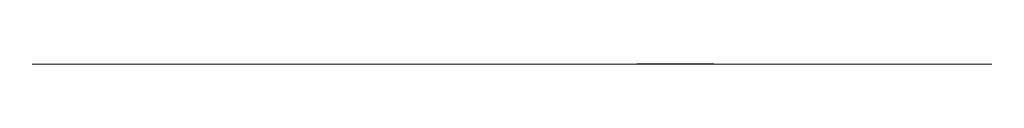
# Model space of a CAD drawing. Units: millimetres. Extents: x 2767 to 3480, y 0 to 1857.
# Tile 1 of 2: x 3181 to 3480, y 0 to 0. Entities that reach past the tile are written whole.
import ezdxf

# ---------------------------------------------------------------- set-up
doc = ezdxf.new("R2010")
doc.units = ezdxf.units.MM
doc.layers.add('M-CONS', color=8, linetype='Continuous', lineweight=18)

# ---------------------------------------------------------------- blocks, each defined once
blk = doc.blocks.new('*U3')
at = {"extrusion": (0, -1, 0)}
blk.add_circle((0, 0), 15.2, dxfattribs=at)
blk = doc.blocks.new('*U4')
at = {"layer": 'M-CONS', "color": 0, "linetype": 'ByBlock', "lineweight": -2, "transparency": 16777216, "extrusion": (-0.866025, 0, 0.5), "rotation": 90}
blk.add_blockref('*U3', (0, 1757.31, -2774.66), dxfattribs=at)
at = {"layer": 'M-CONS', "color": 0, "linetype": 'ByBlock', "lineweight": -2, "transparency": 16777216, "extrusion": (-0.866025, 0, -0.5), "rotation": 90}
blk.add_blockref('*U3', (0, -1572.94, -2881.11), dxfattribs=at)
at = {"layer": 'M-CONS', "color": 0, "linetype": 'ByBlock', "lineweight": -2, "transparency": 16777216}
blk.add_blockref('*U3', (3330.25, 0, 162.64), dxfattribs=at)
at = {"layer": 'M-CONS', "color": 0, "linetype": 'ByBlock', "lineweight": -2, "transparency": 16777216, "extrusion": (-4e-16, 0, -1)}
blk.add_blockref('*U3', (-3330.25, 0, -50.25), dxfattribs=at)
at = {"layer": 'M-CONS', "color": 0, "linetype": 'ByBlock', "lineweight": -2, "transparency": 16777216, "extrusion": (0.866025, 0, -0.5), "rotation": 270}
blk.add_blockref('*U3', (0, 1757.31, 2887.05), dxfattribs=at)
at = {"layer": 'M-CONS', "color": 0, "linetype": 'ByBlock', "lineweight": -2, "transparency": 16777216, "extrusion": (0.866025, 0, 0.5), "rotation": 270}
blk.add_blockref('*U3', (0, -1572.94, 2993.5), dxfattribs=at)
blk = doc.blocks.new('*U5')
at = {"extrusion": (0, -1, 0)}
blk.add_circle((0, 0), 10, dxfattribs=at)
blk = doc.blocks.new('*U6')
at = {"layer": 'M-CONS', "color": 0, "linetype": 'ByBlock', "lineweight": -2, "transparency": 16777216, "extrusion": (-1, 0, -3e-16), "rotation": 90}
blk.add_blockref('*U5', (0, 106.45, -3213.71), dxfattribs=at)
at = {"layer": 'M-CONS', "color": 0, "linetype": 'ByBlock', "lineweight": -2, "transparency": 16777216}
blk.add_blockref('*U5', (3330.25, 0, 222.99), dxfattribs=at)
at = {"layer": 'M-CONS', "color": 0, "linetype": 'ByBlock', "lineweight": -2, "transparency": 16777216, "extrusion": (5e-16, 0, -1)}
blk.add_blockref('*U5', (-3330.25, 0, 10.09), dxfattribs=at)
at = {"layer": 'M-CONS', "color": 0, "linetype": 'ByBlock', "lineweight": -2, "transparency": 16777216, "extrusion": (1, 0, 7e-16), "rotation": 270}
blk.add_blockref('*U5', (0, 106.45, 3446.79), dxfattribs=at)

msp = doc.modelspace()

# ---------------------------------------------------------------- linework, layer by layer
at = {"layer": 'M-CONS', "extrusion": (0, -1, 0)}
for p, q in [((3242.84, 0, 48.18), (3271.99, 0, 19.04)), ((3271.99, 0, 193.86), (3242.84, 0, 164.72)), ((3417.66, 0, 48.18), (3388.52, 0, 19.04)), ((3417.66, 0, 164.72), (3388.52, 0, 193.86))]:
    msp.add_line(p, q, dxfattribs=at)
for radius in [145.68, 87.41, 56.19, 29.14]:
    msp.add_circle((3330.25, 106.45), radius, dxfattribs=at)
for centre, start, end in [((3242.84, 106.45), 70.5305, 289.4695), ((3330.25, 193.86), 340.5305, 199.4695), ((3330.25, 193.86), 340.5305, 199.4695), ((3330.25, 19.04), 160.5305, 19.4695), ((3417.66, 106.45), 250.5305, 109.4695)]:
    msp.add_arc(centre, 58.27, start, end, dxfattribs=at)

# ---------------------------------------------------------------- block references
at = {"layer": 'M-CONS'}
for name in ['*U6', '*U4']:
    msp.add_blockref(name, (0, 0), dxfattribs=at)

doc.saveas('drawing.dxf')
